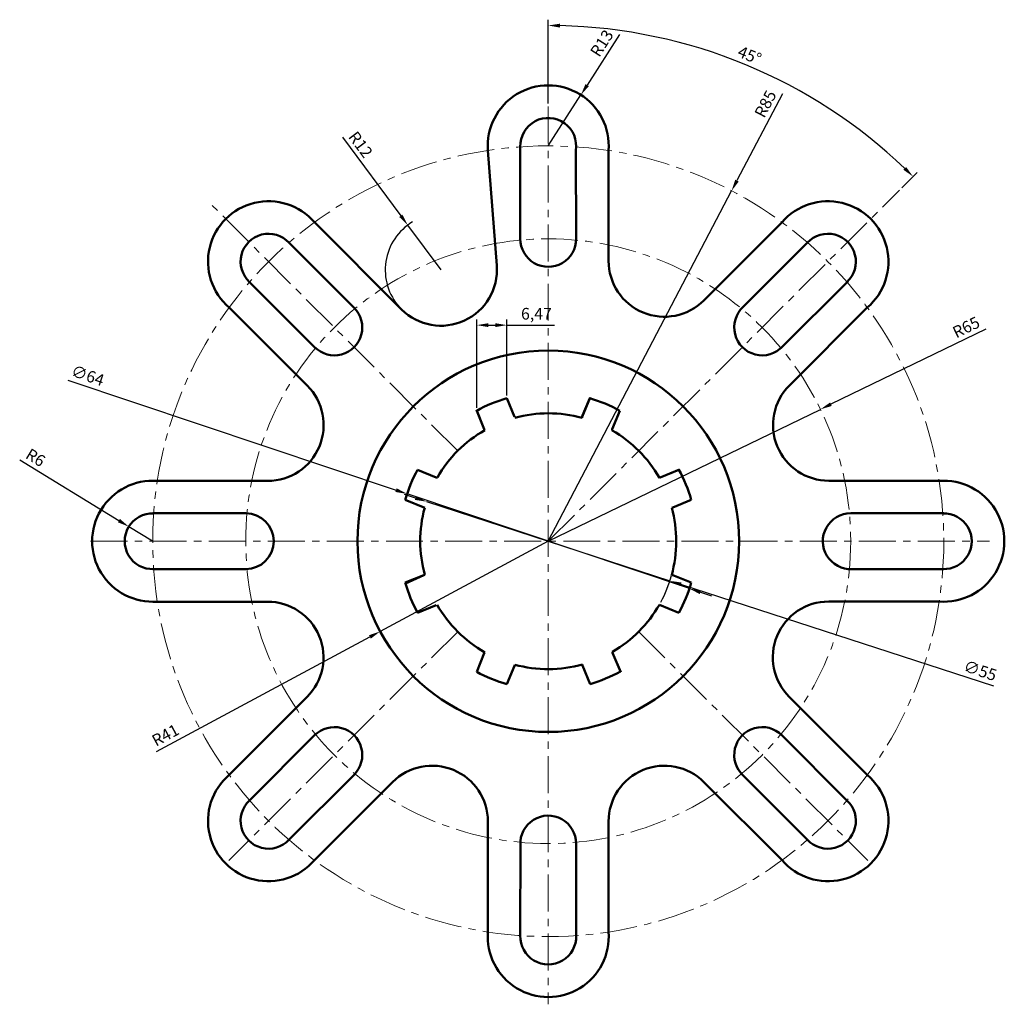
# Model space of a CAD drawing. Units: millimetres. Extents: x 2856 to 3067, y 1297 to 1509.
import ezdxf

# ---------------------------------------------------------------- set-up
doc = ezdxf.new("R2010")
doc.units = ezdxf.units.MM
doc.linetypes.add('CENTER', pattern=[50.8, 31.75, -6.35, 6.35, -6.35])
for name, color, linetype, lineweight in [('M-CNTR', 1, 'CENTER', 18), ('M-DIMS', 2, 'Continuous', 25), ('M-OUTL', 7, 'Continuous', 50)]:
    doc.layers.add(name, color=color, linetype=linetype, lineweight=lineweight)
doc.styles.get("Standard").update_dxf_attribs({"font": 'arial.ttf'})
doc.dimstyles.new('ISO-25', dxfattribs={"dimtxt": 2.5, "dimasz": 2.5, "dimexe": 1.25, "dimexo": 0.625, "dimtad": 1, "dimtxsty": 'Standard', "dimcen": 2.5, "dimadec": 0, "dimazin": 0, "dimtfac": 1, "dimtmove": 0, "dimatfit": 3, "dimfxl": 1, "dimarcsym": 0})

# ---------------------------------------------------------------- blocks, each defined once
blk = doc.blocks.new('*D1')
at = {"layer": 'Defpoints', "color": 0, "transparency": 16777216}
for p in [(2960.53, 1443.31), (2960.53, 1427.59), (2954.06, 1424.92)]:
    blk.add_point(p, dxfattribs=at)
at = {"layer": 'M-DIMS', "color": 0, "lineweight": -2, "transparency": 16777216}
for p, q in [((2954.06, 1425.54), (2954.06, 1444.56)), ((2960.53, 1428.21), (2960.53, 1444.56)), ((2956.56, 1443.31), (2958.03, 1443.31)), ((2960.53, 1443.31), (2970.78, 1443.31))]:
    blk.add_line(p, q, dxfattribs=at)
at = {"layer": 'M-DIMS', "color": 0, "transparency": 16777216}
for points in [[(2956.56, 1443.73), (2956.56, 1442.9), (2954.06, 1443.31)], [(2958.03, 1443.73), (2958.03, 1442.9), (2960.53, 1443.31)]]:
    blk.add_solid(points, dxfattribs=at)
at = {"layer": 'M-DIMS', "color": 0, "transparency": 16777216, "insert": (2966.9, 1445.44), "char_height": 2.5, "attachment_point": 5}
blk.add_mtext('6,47', dxfattribs=at)
blk = doc.blocks.new('*D2')
at = {"layer": 'Defpoints', "color": 0, "transparency": 16777216}
for p in [(2969.43, 1396.85), (2933.31, 1377.46)]:
    blk.add_point(p, dxfattribs=at)
at = {"layer": 'M-DIMS', "color": 0, "lineweight": -2, "transparency": 16777216}
for p, q in [((2969.43, 1396.85), (2933.31, 1377.46)), ((2885.24, 1351.64), (2931.11, 1376.27))]:
    blk.add_line(p, q, dxfattribs=at)
at = {"layer": 'M-DIMS', "color": 0, "transparency": 16777216}
blk.add_solid([(2930.91, 1376.64), (2931.31, 1375.91), (2933.31, 1377.46)], dxfattribs=at)
at = {"layer": 'M-DIMS', "color": 0, "transparency": 16777216, "insert": (2887.32, 1354.89), "char_height": 2.5, "attachment_point": 5, "rotation": 28.2368}
blk.add_mtext('R41', dxfattribs=at)
blk = doc.blocks.new('*D3')
at = {"layer": 'Defpoints', "color": 0, "transparency": 16777216}
for p in [(2879.31, 1399.98), (2884.43, 1396.85)]:
    blk.add_point(p, dxfattribs=at)
at = {"layer": 'M-DIMS', "color": 0, "lineweight": -2, "transparency": 16777216}
for p, q in [((2855.86, 1414.33), (2877.18, 1401.29)), ((2884.43, 1396.85), (2879.31, 1399.98))]:
    blk.add_line(p, q, dxfattribs=at)
at = {"layer": 'M-DIMS', "color": 0, "transparency": 16777216}
blk.add_solid([(2877.4, 1401.64), (2876.96, 1400.93), (2879.31, 1399.98)], dxfattribs=at)
at = {"layer": 'M-DIMS', "color": 0, "transparency": 16777216, "insert": (2859.1, 1414.57), "char_height": 2.5, "attachment_point": 5, "rotation": 328.5525}
blk.add_mtext('R6', dxfattribs=at)
blk = doc.blocks.new('*D4')
at = {"layer": 'Defpoints', "color": 0, "transparency": 16777216}
for p in [(2939.25, 1464.81), (2946.4, 1455.18)]:
    blk.add_point(p, dxfattribs=at)
at = {"layer": 'M-DIMS', "color": 0, "lineweight": -2, "transparency": 16777216}
for p, q in [((2925.19, 1483.72), (2937.75, 1466.82)), ((2946.4, 1455.18), (2939.25, 1464.81))]:
    blk.add_line(p, q, dxfattribs=at)
blk.add_arc((2946.4, 1455.18), 12, 120.6572, 222.0158, dxfattribs=at)
at = {"layer": 'M-DIMS', "color": 0, "transparency": 16777216}
blk.add_solid([(2938.09, 1467.07), (2937.42, 1466.57), (2939.25, 1464.81)], dxfattribs=at)
at = {"layer": 'M-DIMS', "color": 0, "transparency": 16777216, "insert": (2928.85, 1481.95), "char_height": 2.5, "attachment_point": 5, "rotation": 306.6255}
blk.add_mtext('R12', dxfattribs=at)
blk = doc.blocks.new('*D5')
at = {"layer": 'Defpoints', "color": 0, "transparency": 16777216}
for p in [(3008.83, 1472.17), (2969.43, 1396.85)]:
    blk.add_point(p, dxfattribs=at)
at = {"layer": 'M-DIMS', "color": 0, "lineweight": -2, "transparency": 16777216}
for p, q in [((3019.75, 1493.06), (3009.99, 1474.39)), ((2969.43, 1396.85), (3008.83, 1472.17))]:
    blk.add_line(p, q, dxfattribs=at)
at = {"layer": 'M-DIMS', "color": 0, "transparency": 16777216}
blk.add_solid([(3009.62, 1474.58), (3010.36, 1474.19), (3008.83, 1472.17)], dxfattribs=at)
at = {"layer": 'M-DIMS', "color": 0, "transparency": 16777216, "insert": (3016.39, 1490.73), "char_height": 2.5, "attachment_point": 5, "rotation": 62.3879}
blk.add_mtext('R85', dxfattribs=at)
blk = doc.blocks.new('*D6')
at = {"layer": 'Defpoints', "color": 0, "transparency": 16777216}
for p in [(2976.45, 1492.8), (2969.43, 1481.85)]:
    blk.add_point(p, dxfattribs=at)
at = {"layer": 'M-DIMS', "color": 0, "lineweight": -2, "transparency": 16777216}
for p, q in [((2984.76, 1505.78), (2977.79, 1494.9)), ((2969.43, 1481.85), (2976.45, 1492.8))]:
    blk.add_line(p, q, dxfattribs=at)
at = {"layer": 'M-DIMS', "color": 0, "transparency": 16777216}
blk.add_solid([(2977.44, 1495.13), (2978.15, 1494.68), (2976.45, 1492.8)], dxfattribs=at)
at = {"layer": 'M-DIMS', "color": 0, "transparency": 16777216, "insert": (2981.21, 1503.76), "char_height": 2.5, "attachment_point": 5, "rotation": 57.3497}
blk.add_mtext('R13', dxfattribs=at)
blk = doc.blocks.new('*D7')
at = {"layer": 'Defpoints', "color": 0, "transparency": 16777216}
for p in [(3027.92, 1425.21), (2969.43, 1396.85)]:
    blk.add_point(p, dxfattribs=at)
at = {"layer": 'M-DIMS', "color": 0, "lineweight": -2, "transparency": 16777216}
for p, q in [((3063.47, 1442.45), (3030.17, 1426.3)), ((2969.43, 1396.85), (3027.92, 1425.21))]:
    blk.add_line(p, q, dxfattribs=at)
at = {"layer": 'M-DIMS', "color": 0, "transparency": 16777216}
blk.add_solid([(3029.99, 1426.68), (3030.35, 1425.93), (3027.92, 1425.21)], dxfattribs=at)
at = {"layer": 'M-DIMS', "color": 0, "transparency": 16777216, "insert": (3059.38, 1442.58), "char_height": 2.5, "attachment_point": 5, "rotation": 25.8689}
blk.add_mtext('R65', dxfattribs=at)
blk = doc.blocks.new('*D8')
at = {"layer": 'Defpoints', "color": 0, "transparency": 16777216}
for p in [(2939.1, 1407.04), (2999.77, 1386.67)]:
    blk.add_point(p, dxfattribs=at)
at = {"layer": 'M-DIMS', "color": 0, "lineweight": -2, "transparency": 16777216}
for p, q in [((2866.18, 1431.51), (2936.73, 1407.83)), ((2999.77, 1386.67), (2939.1, 1407.04)), ((3002.14, 1385.88), (3004.51, 1385.08))]:
    blk.add_line(p, q, dxfattribs=at)
at = {"layer": 'M-DIMS', "color": 0, "transparency": 16777216}
for points in [[(2936.86, 1408.23), (2936.59, 1407.44), (2939.1, 1407.04)], [(3002.27, 1386.27), (3002.01, 1385.48), (2999.77, 1386.67)]]:
    blk.add_solid(points, dxfattribs=at)
at = {"layer": 'M-DIMS', "color": 0, "transparency": 16777216, "insert": (2870.38, 1432.18), "char_height": 2.5, "attachment_point": 5, "rotation": 341.4479}
blk.add_mtext('∅64', dxfattribs=at)
blk = doc.blocks.new('*D9')
at = {"layer": 'Defpoints', "color": 0, "transparency": 16777216}
for p in [(2943.28, 1405.37), (2995.58, 1388.34)]:
    blk.add_point(p, dxfattribs=at)
at = {"layer": 'M-DIMS', "color": 0, "lineweight": -2, "transparency": 16777216}
for p, q in [((2940.91, 1406.14), (2938.53, 1406.91)), ((2943.28, 1405.37), (2995.58, 1388.34)), ((3065.15, 1365.69), (2997.96, 1387.57))]:
    blk.add_line(p, q, dxfattribs=at)
blk.add_arc((2969.43, 1396.85), 27.5, 331.5493, 344.5729, dxfattribs=at)
at = {"layer": 'M-DIMS', "color": 0, "transparency": 16777216}
for points in [[(2941.03, 1406.54), (2940.78, 1405.74), (2943.28, 1405.37)], [(2998.09, 1387.96), (2997.83, 1387.17), (2995.58, 1388.34)]]:
    blk.add_solid(points, dxfattribs=at)
at = {"layer": 'M-DIMS', "color": 0, "transparency": 16777216, "insert": (3062.16, 1368.74), "char_height": 2.5, "attachment_point": 5, "rotation": 341.9685}
blk.add_mtext('∅55', dxfattribs=at)
blk = doc.blocks.new('*D10')
at = {"layer": 'Defpoints', "color": 0, "transparency": 16777216}
for p in [(3024.87, 1492.88), (2969.43, 1490.32), (3044.94, 1472.36), (2969.43, 1396.85), (2969.43, 1297.29)]:
    blk.add_point(p, dxfattribs=at)
at = {"layer": 'M-DIMS', "color": 0, "lineweight": -2, "transparency": 16777216}
for p, q in [((2969.43, 1490.94), (2969.43, 1508.98)), ((3045.38, 1472.8), (3048.72, 1476.14))]:
    blk.add_line(p, q, dxfattribs=at)
blk.add_arc((2969.43, 1396.85), 110.88, 46.2919, 88.7081, dxfattribs=at)
at = {"layer": 'M-DIMS', "color": 0, "transparency": 16777216}
for points in [[(2971.93, 1507.29), (2971.94, 1508.12), (2969.43, 1507.73)], [(3046.34, 1477.3), (3045.76, 1476.71), (3047.83, 1475.26)]]:
    blk.add_solid(points, dxfattribs=at)
at = {"layer": 'M-DIMS', "color": 0, "transparency": 16777216, "insert": (3012.59, 1501.04), "char_height": 2.5, "attachment_point": 5, "rotation": 337.5}
blk.add_mtext('45°', dxfattribs=at)

msp = doc.modelspace()

# ---------------------------------------------------------------- linework, layer by layer
at = {"layer": 'M-CNTR', "ltscale": 0.25, "transparency": 33554534}
for p, q in [((2969.432, 1490.318), (2969.432, 1297.294)), ((2969.432, 1396.854), (3044.939, 1472.361)), ((2949.987, 1416.299), (2896.644, 1469.642)), ((2871.079, 1396.854), (3064.287, 1396.854)), ((2949.987, 1377.408), (2900.783, 1328.205)), ((2988.878, 1377.408), (3038.081, 1328.205))]:
    msp.add_line(p, q, dxfattribs=at)
for radius in [85, 65]:
    msp.add_circle((2969.432, 1396.854), radius, dxfattribs=at)
at = {"layer": 'M-OUTL'}
for p, q in [((2963.432, 1481.854), (2963.432, 1461.854)), ((2956.47, 1480.86), (2958.369, 1456.101)), ((2975.349, 1480.86), (2975.432, 1461.88)), ((2982.394, 1480.86), (2982.394, 1457.117)), ((2919.197, 1465.42), (2937.919, 1446.698)), ((3019.668, 1465.42), (3002.879, 1448.632)), ((2913.718, 1461.048), (2927.712, 1447.059)), ((3010.96, 1446.858), (3025.292, 1461.199)), ((2905.238, 1452.568), (2919.227, 1438.574)), ((3019.436, 1438.382), (3033.778, 1452.714)), ((2900.866, 1447.089), (2917.65, 1430.305)), ((3037.999, 1447.089), (3021.248, 1430.339)), ((3037.999, 1447.089), (3037.999, 1447.089)), ((2962.17, 1423.607), (2960.525, 1427.589)), ((2976.609, 1423.401), (2978.339, 1427.589)), ((2976.695, 1423.607), (2978.413, 1427.767)), ((2955.7, 1420.935), (2953.982, 1425.094)), ((2954.055, 1424.917), (2955.7, 1420.935)), ((2983.165, 1420.935), (2984.809, 1424.917)), ((2976.695, 1423.607), (2976.695, 1423.377)), ((2955.785, 1420.728), (2955.7, 1420.935)), ((2983.165, 1420.935), (2983.165, 1420.679)), ((2945.351, 1410.586), (2941.369, 1412.231)), ((2993.514, 1410.586), (2997.673, 1412.304)), ((2993.514, 1410.586), (2997.495, 1412.231)), ((2884.432, 1409.854), (2909.148, 1409.82)), ((2945.351, 1410.586), (2945.606, 1410.586)), ((2993.514, 1410.586), (2993.307, 1410.501)), ((3054.432, 1409.854), (3029.734, 1409.854)), ((2942.885, 1404.031), (2938.697, 1405.761)), ((2996.186, 1404.116), (3000.168, 1405.761)), ((2996.186, 1404.116), (2995.979, 1404.031)), ((2884.432, 1402.854), (2904.432, 1402.854)), ((3034.432, 1402.854), (3054.432, 1402.854)), ((2884.432, 1390.854), (2904.432, 1390.854)), ((3034.155, 1390.86), (3054.432, 1390.854)), ((2942.679, 1389.591), (2938.697, 1387.947)), ((2942.679, 1389.591), (2938.758, 1387.74)), ((2942.679, 1389.591), (2942.893, 1389.649)), ((2996.186, 1389.591), (2995.956, 1389.591)), ((2996.186, 1389.591), (3000.168, 1387.947)), ((2884.432, 1383.854), (2909.131, 1383.854)), ((2945.351, 1383.121), (2941.369, 1381.477)), ((2993.307, 1383.207), (2997.495, 1381.477)), ((3053.438, 1383.892), (3029.696, 1383.892)), ((2955.7, 1372.772), (2954.055, 1368.79)), ((2955.7, 1372.772), (2955.81, 1372.965)), ((2983.264, 1372.829), (2983.264, 1373.085)), ((2983.264, 1372.829), (2984.925, 1368.854)), ((2983.264, 1372.829), (2984.999, 1368.677)), ((2962.17, 1370.1), (2960.525, 1366.118)), ((2962.17, 1370.1), (2962.228, 1370.314)), ((2976.805, 1370.13), (2976.805, 1370.361)), ((2976.805, 1370.13), (2978.466, 1366.155)), ((2900.866, 1346.618), (2917.616, 1363.368)), ((3037.999, 1346.618), (3021.21, 1363.406)), ((2905.238, 1341.139), (2919.227, 1355.134)), ((3033.627, 1341.139), (3019.638, 1355.134)), ((2913.718, 1332.659), (2927.712, 1346.648)), ((3025.147, 1332.659), (3010.96, 1346.849)), ((2919.197, 1328.287), (2935.985, 1345.076)), ((3019.668, 1328.287), (3002.879, 1345.076)), ((2956.47, 1312.848), (2956.47, 1336.59)), ((2982.394, 1312.848), (2982.394, 1336.59)), ((2963.436, 1312.065), (2963.439, 1332.131)), ((2975.428, 1312.065), (2975.432, 1331.853)), ((2969.432, 1297.294), (2969.432, 1297.294))]:
    msp.add_line(p, q, dxfattribs=at)
msp.add_circle((2969.432, 1396.854), 41, dxfattribs=at)
for centre, radius, start, end in [((2969.432, 1481.854), 13, 355.61428, 184.38572), ((2969.432, 1481.854), 6, 350.4629, 182.02262), ((2909.328, 1456.958), 13, 40.61428, 229.38572), ((3029.536, 1456.958), 13, 310.61428, 139.38572), ((2909.328, 1456.958), 6, 42.97738, 227.02262), ((3029.536, 1456.958), 6, 312.97738, 137.02262), ((2969.432, 1461.854), 6, 180, 0.25017), ((2994.394, 1457.117), 12, 180, 315), ((2946.404, 1455.183), 12, 225, 4.38574), ((2923.47, 1442.816), 6, 224.98918, 45.01082), ((3015.394, 1442.816), 6, 132.39078, 317.60922), ((2909.164, 1421.82), 12, 269.92172, 45), ((3029.734, 1421.854), 12, 135, 270), ((2969.432, 1396.854), 32, 106.16157, 118.72015), ((2969.432, 1396.854), 32, 61.27985, 73.83843), ((2969.432, 1396.854), 27.5, 74.68683, 105.14235), ((2969.432, 1396.854), 27.5, 119.75288, 150.04204), ((2969.432, 1396.854), 27.5, 29.75288, 60.04204), ((2969.432, 1396.854), 32, 151.27985, 163.83843), ((2969.432, 1396.854), 32, 16.16157, 28.72015), ((2884.432, 1396.854), 13, 85.61428, 274.38572), ((3054.432, 1396.854), 13, 265.61428, 94.38572), ((2969.432, 1396.854), 27.5, 164.87116, 195.18767), ((2969.432, 1396.854), 27.5, 344.68683, 15.12884), ((2884.432, 1396.854), 6, 87.97738, 272.02262), ((2904.432, 1396.854), 6, 270, 90), ((3034.432, 1396.854), 6, 90, 272.60923), ((3054.432, 1396.854), 6, 267.97738, 92.02262), ((2969.432, 1396.854), 32, 196.16157, 208.72015), ((2969.432, 1396.854), 32, 331.27985, 343.83843), ((2909.131, 1371.854), 12, 315, 90), ((2969.432, 1396.854), 27.5, 209.75288, 240.30595), ((2969.432, 1396.854), 27.5, 300.19707, 330.24712), ((3029.696, 1371.892), 12, 90, 225), ((2969.432, 1396.854), 27.5, 254.81233, 285.55178), ((2969.432, 1396.854), 32, 241.27985, 253.83843), ((2969.432, 1396.854), 32, 286.39813, 298.95671), ((2923.47, 1350.892), 6, 314.98918, 135.01082), ((3015.394, 1350.892), 6, 44.98918, 227.63019), ((2944.47, 1336.59), 12, 0, 135), ((2994.394, 1336.59), 12, 45, 180), ((2909.328, 1336.75), 13, 130.61428, 319.38572), ((3029.536, 1336.75), 13, 220.61428, 49.38572), ((2909.328, 1336.75), 6, 132.97738, 317.02262), ((3029.536, 1336.75), 6, 222.97738, 47.02262), ((2969.432, 1331.854), 6, 359.98918, 182.63019), ((2969.432, 1311.854), 13, 175.61428, 4.38572), ((2969.432, 1311.854), 6, 177.97738, 2.02262)]:
    msp.add_arc(centre, radius, start, end, dxfattribs=at)

# ---------------------------------------------------------------- dimensions: what is measured, and where the dimension line sits
at = {"layer": 'M-DIMS'}
dim = msp.add_angular_dim_2l(base=(3024.871, 1492.877), line1=((2969.432, 1396.854), (3044.939, 1472.361)), line2=((2969.432, 1490.318), (2969.432, 1297.294)), dimstyle='ISO-25', override={"dimclrd": 0, "dimclre": 0, "dimclrt": 0}, dxfattribs=at)
dim.commit()
dim.dimension.update_dxf_attribs({"geometry": '*D10', "text_midpoint": (3012.589, 1501.043)})
for center, mpoint, picture, middle in [((2969.432, 1481.854), (2976.446, 1492.799), '*D6', (2982.813, 1502.736)), ((2969.432, 1396.854), (3008.828, 1472.173), '*D5', (3018.073, 1489.848)), ((2946.404, 1455.183), (2939.245, 1464.814), '*D4', (2927.342, 1480.827)), ((2969.432, 1396.854), (3027.919, 1425.214), '*D7', (3060.214, 1440.874)), ((2884.432, 1396.854), (2879.314, 1399.984), '*D3', (2858.111, 1412.95)), ((2969.432, 1396.854), (2933.311, 1377.456), '*D2', (2888.211, 1353.236))]:
    dim = msp.add_radius_dim(center=center, mpoint=mpoint, dimstyle='ISO-25', override={"dimclrd": 0, "dimclre": 0, "dimclrt": 0}, dxfattribs=at)
    dim.commit()
    dim.dimension.update_dxf_attribs({"geometry": picture, "text_midpoint": middle, "dimtype": 164})
dim = msp.add_linear_dim(base=(2960.525, 1443.313), p1=(2954.055, 1424.917), p2=(2960.525, 1427.589), dimstyle='ISO-25', override={"dimclrd": 0, "dimclre": 0, "dimclrt": 0}, dxfattribs=at)
dim.commit()
dim.dimension.update_dxf_attribs({"geometry": '*D1', "text_midpoint": (2966.904, 1445.44)})
for p1, p2, picture, middle in [((2999.769, 1386.672), (2939.095, 1407.035), '*D8', (2869.751, 1430.307)), ((2943.283, 1405.366), (2995.582, 1388.341), '*D9', (3061.551, 1366.866))]:
    dim = msp.add_diameter_dim_2p(p1=p1, p2=p2, dimstyle='ISO-25', override={"dimclrd": 0, "dimclre": 0, "dimclrt": 0}, dxfattribs=at)
    dim.commit()
    dim.dimension.update_dxf_attribs({"geometry": picture, "text_midpoint": middle, "dimtype": 163})

doc.saveas('drawing.dxf')
